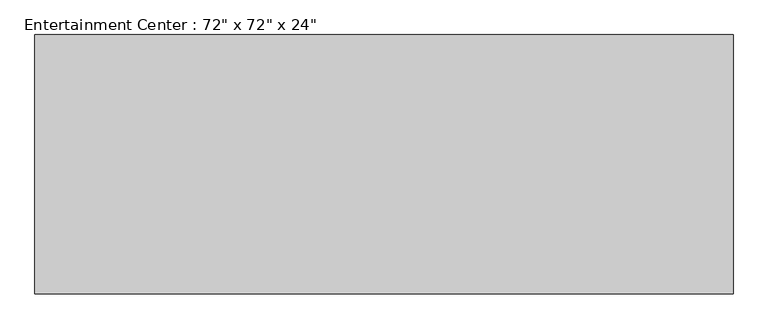
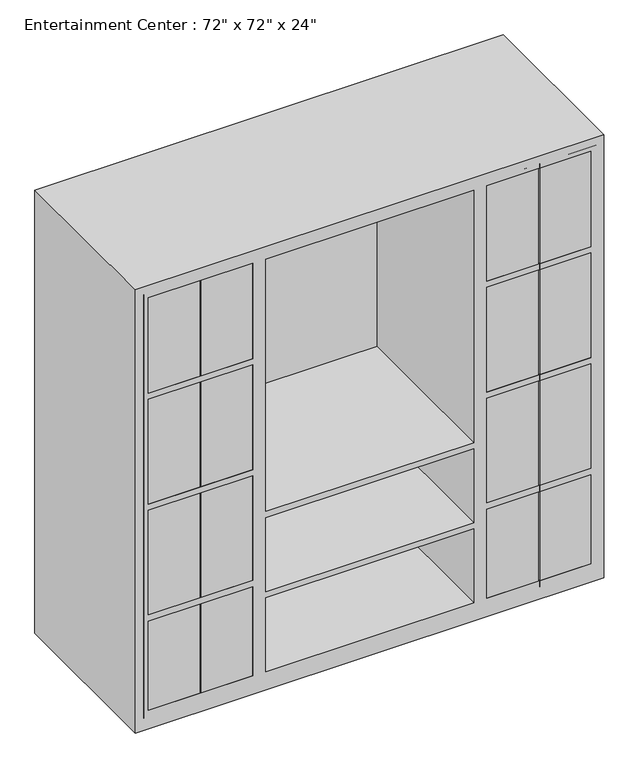
"""IFC4 building model written with IfcOpenShell, lengths in millimetres: furniture geometry."""

from ifc_helpers import new_model, si_unit, point, frame, frame_2d, origin, place, context, project, spatial, polyline, circle_curve, trimmed, segment, composite_curve, outline, extrude, faceted_brep, source, transform, mapped, element, save


def furniture_cf0b6580(model_context):
    return source(origin(), model_context, "Body", "SolidModel", [
        faceted_brep([(914.4, -781.05, 0.0), (914.4, -781.05, 1828.8), (-914.4, -781.05, 1828.8), (-914.4, -781.05, 0.0), (-457.2, -781.05, 1778.0), (-457.2, -781.05, 1384.3), (-863.6, -781.05, 1384.3), (-863.6, -781.05, 1778.0), (-457.2, -781.05, 76.2), (-863.6, -781.05, 76.2), (-863.6, -781.05, 444.5), (-457.2, -781.05, 444.5), (863.6, -781.05, 1384.3), (457.2, -781.05, 1384.3), (457.2, -781.05, 1778.0), (863.6, -781.05, 1778.0), (-406.4, -781.05, 736.6), (-406.4, -781.05, 1778.0), (406.4, -781.05, 1778.0), (406.4, -781.05, 736.6), (406.4, -781.05, 76.2), (-406.4, -781.05, 76.2), (-406.4, -781.05, 381.0), (406.4, -781.05, 381.0), (863.6, -781.05, 76.2), (457.2, -781.05, 76.2), (457.2, -781.05, 444.5), (863.6, -781.05, 444.5), (-863.6, -781.05, 469.9), (-863.6, -781.05, 901.7), (-457.2, -781.05, 901.7), (-457.2, -781.05, 469.9), (-457.2, -781.05, 1358.9), (-457.2, -781.05, 927.1), (-863.6, -781.05, 927.1), (-863.6, -781.05, 1358.9), (457.2, -781.05, 1358.9), (863.6, -781.05, 1358.9), (863.6, -781.05, 927.1), (457.2, -781.05, 927.1), (457.2, -781.05, 901.7), (863.6, -781.05, 901.7), (863.6, -781.05, 469.9), (457.2, -781.05, 469.9), (406.4, -781.05, 406.4), (-406.4, -781.05, 406.4), (-406.4, -781.05, 711.2), (406.4, -781.05, 711.2), (914.4, -101.6, 0.0), (-914.4, -101.6, 0.0), (-914.4, -101.6, 1828.8), (914.4, -101.6, 1828.8), (-457.2, -127.0, 1778.0), (-457.2, -127.0, 1384.3), (-863.6, -127.0, 1384.3), (-863.6, -127.0, 1778.0), (-457.2, -127.0, 76.2), (-863.6, -127.0, 76.2), (-863.6, -127.0, 444.5), (-457.2, -127.0, 444.5), (863.6, -127.0, 1384.3), (457.2, -127.0, 1384.3), (457.2, -127.0, 1778.0), (863.6, -127.0, 1778.0), (-406.4, -127.0, 736.6), (-406.4, -127.0, 1778.0), (406.4, -127.0, 1778.0), (406.4, -127.0, 736.6), (406.4, -127.0, 76.2), (-406.4, -127.0, 76.2), (-406.4, -127.0, 381.0), (406.4, -127.0, 381.0), (863.6, -127.0, 76.2), (457.2, -127.0, 76.2), (457.2, -127.0, 444.5), (863.6, -127.0, 444.5), (-863.6, -127.0, 469.9), (-863.6, -127.0, 901.7), (-457.2, -127.0, 901.7), (-457.2, -127.0, 469.9), (-457.2, -127.0, 1358.9), (-457.2, -127.0, 927.1), (-863.6, -127.0, 927.1), (-863.6, -127.0, 1358.9), (457.2, -127.0, 1358.9), (863.6, -127.0, 1358.9), (863.6, -127.0, 927.1), (457.2, -127.0, 927.1), (457.2, -127.0, 901.7), (863.6, -127.0, 901.7), (863.6, -127.0, 469.9), (457.2, -127.0, 469.9), (406.4, -127.0, 406.4), (-406.4, -127.0, 406.4), (-406.4, -127.0, 711.2), (406.4, -127.0, 711.2)], [[[0, 1, 2, 3], [4, 5, 6, 7], [8, 9, 10, 11], [12, 13, 14, 15], [16, 17, 18, 19], [20, 21, 22, 23], [24, 25, 26, 27], [28, 29, 30, 31], [32, 33, 34, 35], [36, 37, 38, 39], [40, 41, 42, 43], [44, 45, 46, 47]], [[48, 49, 50, 51]], [[1, 0, 48, 51]], [[2, 1, 51, 50]], [[3, 2, 50, 49]], [[0, 3, 49, 48]], [[5, 4, 52, 53]], [[6, 5, 53, 54]], [[7, 6, 54, 55]], [[4, 7, 55, 52]], [[9, 8, 56, 57]], [[10, 9, 57, 58]], [[11, 10, 58, 59]], [[8, 11, 59, 56]], [[13, 12, 60, 61]], [[14, 13, 61, 62]], [[15, 14, 62, 63]], [[12, 15, 63, 60]], [[17, 16, 64, 65]], [[18, 17, 65, 66]], [[19, 18, 66, 67]], [[16, 19, 67, 64]], [[21, 20, 68, 69]], [[22, 21, 69, 70]], [[23, 22, 70, 71]], [[20, 23, 71, 68]], [[25, 24, 72, 73]], [[26, 25, 73, 74]], [[27, 26, 74, 75]], [[24, 27, 75, 72]], [[29, 28, 76, 77]], [[30, 29, 77, 78]], [[31, 30, 78, 79]], [[28, 31, 79, 76]], [[33, 32, 80, 81]], [[34, 33, 81, 82]], [[35, 34, 82, 83]], [[32, 35, 83, 80]], [[37, 36, 84, 85]], [[38, 37, 85, 86]], [[39, 38, 86, 87]], [[36, 39, 87, 84]], [[41, 40, 88, 89]], [[42, 41, 89, 90]], [[43, 42, 90, 91]], [[40, 43, 91, 88]], [[45, 44, 92, 93]], [[46, 45, 93, 94]], [[47, 46, 94, 95]], [[44, 47, 95, 92]], [[53, 52, 55, 54]], [[57, 56, 59, 58]], [[61, 60, 63, 62]], [[65, 64, 67, 66]], [[69, 68, 71, 70]], [[73, 72, 75, 74]], [[77, 76, 79, 78]], [[81, 80, 83, 82]], [[85, 84, 87, 86]], [[89, 88, 91, 90]], [[93, 92, 95, 94]]]),
        extrude(outline(composite_curve([segment(polyline([(1003.3, -632.9986452), (1003.3, -657.225), (825.5, -657.225), (825.5, -632.9986452)]), True, "CONTINUOUS"), segment(trimmed(circle_curve(frame_2d((850.9, -632.9986452)), 25.4), [point((825.5, -632.9986452))], [point((850.9, -607.5986452))], False, "CARTESIAN"), True, "CONTINUOUS"), segment(polyline([(850.9, -607.5986452), (977.9, -607.5986452)]), True, "CONTINUOUS"), segment(trimmed(circle_curve(frame_2d((977.9, -632.9986452)), 25.4), [point((977.9, -607.5986452))], [point((1003.3, -632.9986452))], False, "CARTESIAN"), True, "CONTINUOUS")], self_intersect=False)), frame((0.0, -714.375, 0.0), z_axis=(0.0, 1.0, 0.0), x_axis=(0.0, 0.0, 1.0)), (0.0, 0.0, 1.0), 3.175),
        extrude(outline(composite_curve([segment(trimmed(circle_curve(frame_2d((977.9, -688.18125)), 25.4), [point((1003.3, -688.18125))], [point((977.9, -713.58125))], False, "CARTESIAN"), True, "CONTINUOUS"), segment(polyline([(977.9, -713.58125), (850.9, -713.58125)]), True, "CONTINUOUS"), segment(trimmed(circle_curve(frame_2d((850.9, -688.18125)), 25.4), [point((850.9, -713.58125))], [point((825.5, -688.18125))], False, "CARTESIAN"), True, "CONTINUOUS"), segment(polyline([(825.5, -688.18125), (825.5, -663.575), (1003.3, -663.575), (1003.3, -688.18125)]), True, "CONTINUOUS")], self_intersect=False)), frame((0.0, -714.375, 0.0), z_axis=(0.0, 1.0, 0.0), x_axis=(0.0, 0.0, 1.0)), (0.0, 0.0, 1.0), 3.175),
        extrude(outline(composite_curve([segment(trimmed(circle_curve(frame_2d((977.9, 632.9986452)), 25.4), [point((1003.3, 632.9986452))], [point((977.9, 607.5986452))], False, "CARTESIAN"), True, "CONTINUOUS"), segment(polyline([(977.9, 607.5986452), (850.9, 607.5986452)]), True, "CONTINUOUS"), segment(trimmed(circle_curve(frame_2d((850.9, 632.9986452)), 25.4), [point((850.9, 607.5986452))], [point((825.5, 632.9986452))], False, "CARTESIAN"), True, "CONTINUOUS"), segment(polyline([(825.5, 632.9986452), (825.5, 657.225), (1003.3, 657.225), (1003.3, 632.9986452)]), True, "CONTINUOUS")], self_intersect=False)), frame((0.0, -714.375, 0.0), z_axis=(0.0, 1.0, 0.0), x_axis=(0.0, 0.0, 1.0)), (0.0, 0.0, 1.0), 3.175),
        extrude(outline(composite_curve([segment(polyline([(1003.3, 688.18125), (1003.3, 663.575), (825.5, 663.575), (825.5, 688.18125)]), True, "CONTINUOUS"), segment(trimmed(circle_curve(frame_2d((850.9, 688.18125)), 25.4), [point((825.5, 688.18125))], [point((850.9, 713.58125))], False, "CARTESIAN"), True, "CONTINUOUS"), segment(polyline([(850.9, 713.58125), (977.9, 713.58125)]), True, "CONTINUOUS"), segment(trimmed(circle_curve(frame_2d((977.9, 688.18125)), 25.4), [point((977.9, 713.58125))], [point((1003.3, 688.18125))], False, "CARTESIAN"), True, "CONTINUOUS")], self_intersect=False)), frame((0.0, -714.375, 0.0), z_axis=(0.0, 1.0, 0.0), x_axis=(0.0, 0.0, 1.0)), (0.0, 0.0, 1.0), 3.175),
        extrude(outline(polyline([(-882.65, -711.2), (-663.575, -711.2), (-663.575, -781.05), (-882.65, -781.05), (-882.65, -711.2)])), frame((0.0, 0.0, 50.8), z_axis=(0.0, 0.0, 1.0), x_axis=(1.0, 0.0, 0.0)), (0.0, 0.0, 1.0), 1746.25),
        extrude(outline(polyline([(-657.225, -711.2), (-438.15, -711.2), (-438.15, -781.05), (-657.225, -781.05), (-657.225, -711.2)])), frame((0.0, 0.0, 50.8), z_axis=(0.0, 0.0, 1.0), x_axis=(1.0, 0.0, 0.0)), (0.0, 0.0, 1.0), 1746.25),
        extrude(outline(polyline([(663.575, -711.2), (882.65, -711.2), (882.65, -781.05), (663.575, -781.05), (663.575, -711.2)])), frame((0.0, 0.0, 50.8), z_axis=(0.0, 0.0, 1.0), x_axis=(1.0, 0.0, 0.0)), (0.0, 0.0, 1.0), 1746.25),
        extrude(outline(polyline([(438.15, -711.2), (657.225, -711.2), (657.225, -781.05), (438.15, -781.05), (438.15, -711.2)])), frame((0.0, 0.0, 50.8), z_axis=(0.0, 0.0, 1.0), x_axis=(1.0, 0.0, 0.0)), (0.0, 0.0, 1.0), 1746.25),
    ])


if __name__ == "__main__":
    model = new_model("IFC4")
    model_context = context("Model", 3, world=origin())
    ifc_project = project(units=[si_unit("LENGTHUNIT", "METRE", prefix="MILLI")], contexts=[model_context])
    site = spatial("IfcSite", under=ifc_project)
    building = spatial("IfcBuilding", under=site)
    placement = place(None, origin())
    furniture_shape = furniture_cf0b6580(model_context)
    element("IfcFurniture", 1, ObjectType="Entertainment Center : 72\" x 72\" x 24\"", at=placement, inside=building, context=model_context, shape_type="MappedRepresentation", body=[
        mapped(furniture_shape, transform((0.0, 0.0, 0.0), x_axis=(1.0, 0.0, 0.0), y_axis=(0.0, 1.0, 0.0), z_axis=(0.0, 0.0, 1.0))),
    ])
    save(model, "model.ifc")

# Revit data of these elements
# Type "Entertainment Center : 72\" x 72\" x 24\""
#   Assembly Code = "E2020200"
#   Center Width = 2' - 8"
#   Depth = 2' - 0"
#   Height = 6' - 0"
#   Width = 6' - 0"
#   Material = Porcelain, Linen
#   Default Elevation = 0
# Element 1 (IfcFurniture, "Entertainment Center : 72\" x 72\" x 24\"")
#   Materials on its faces: "Porcelain, Linen", "Steel, Chrome Plated", "Glass - Clear, Grey"
# Materials
#   "Porcelain, Linen": class "Ceramic", colour RGB 249 239 230, transparency 0, Description = "Porcelain, linen", Cost = 0
#   "Steel, Chrome Plated": class "Metal", colour RGB 17 17 17, transparency 0, Description = "Chromiuim plated steel", Cost = 0
#   "Glass - Clear, Grey": class "Glass", colour RGB 252 255 255, transparency 0.64
